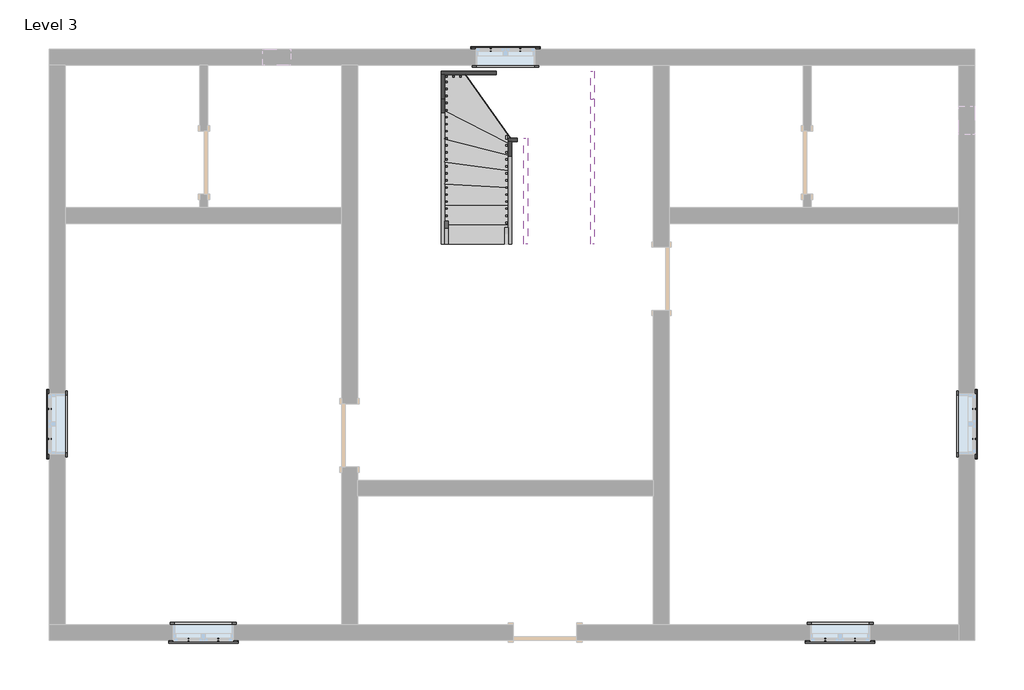
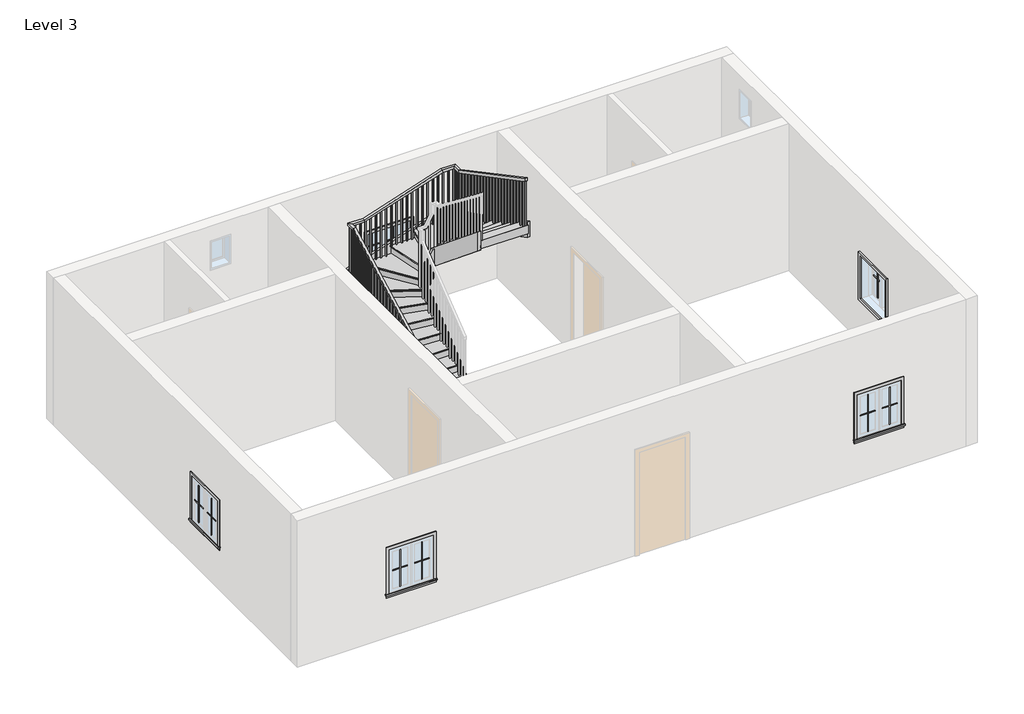
# One storey, part 2 of 2: 20 proxies, 8 members, 1 railing, 1 stair flight.
"""IFC4 building model written with IfcOpenShell, lengths in millimetres."""

from ifc_helpers import new_model, si_unit, frame, origin, place, context, project, spatial, polyline, outline, extrude, faceted_brep, transform, mapped, element, save
from components import muntin_pattern_2x2_muntin_pattern_2x2_b3fe6957, muntin_pattern_2x2_muntin_pattern_2x2_3e0ecaf2, trim_window_exterior_flat_with_sill_41619996, trim_window_interior_flat_picture_frame_51c85655, stair_flight_4b86e887

model = new_model("IFC4")

# Units and contexts
model_context = context("Model", 3, world=origin())
ifc_project = project(units=[si_unit("LENGTHUNIT", "METRE", prefix="MILLI")], contexts=[model_context])

# Site, building, storey
site = spatial("IfcSite", under=ifc_project)
building = spatial("IfcBuilding", under=site)
storey = spatial("IfcBuildingStorey", under=building, Name="Level 3", Elevation=3200.4)

# Proxies
placement = place(None, origin())
muntin_pattern_2x2_muntin_pattern_2x2_shape = muntin_pattern_2x2_muntin_pattern_2x2_b3fe6957(model_context)
element("IfcBuildingElementProxy", 1, Name="Muntin Pattern_2x2 : Muntin Pattern_2x2", ObjectType="Muntin Pattern_2x2 : Muntin Pattern_2x2", at=placement, inside=storey, context=model_context, shape_type="MappedRepresentation", body=[
    mapped(muntin_pattern_2x2_muntin_pattern_2x2_shape, transform((-7325.4390964, 833.891032, 4184.65), x_axis=(0.0, 1.0, 0.0), y_axis=(-1.0, 0.0, 0.0), z_axis=(0.0, 0.0, 1.0))),
])
element("IfcBuildingElementProxy", 2, Name="Muntin Pattern_2x2 : Muntin Pattern_2x2", ObjectType="Muntin Pattern_2x2 : Muntin Pattern_2x2", at=placement, inside=storey, context=model_context, shape_type="MappedRepresentation", body=[
    mapped(muntin_pattern_2x2_muntin_pattern_2x2_shape, transform((6006.3859036, 1262.516032, 4184.65), x_axis=(0.0, -1.0, 0.0), y_axis=(1.0, 0.0, 0.0), z_axis=(0.0, 0.0, 1.0))),
])
element("IfcBuildingElementProxy", 3, Name="Muntin Pattern_2x2 : Muntin Pattern_2x2", ObjectType="Muntin Pattern_2x2 : Muntin Pattern_2x2", at=placement, inside=storey, context=model_context, shape_type="MappedRepresentation", body=[
    mapped(muntin_pattern_2x2_muntin_pattern_2x2_shape, transform((-967.5015964, 6448.878532, 4184.65), x_axis=(1.0, 0.0, 0.0), y_axis=(0.0, 1.0, 0.0), z_axis=(0.0, 0.0, 1.0))),
])
element("IfcBuildingElementProxy", 4, Name="Muntin Pattern_2x2 : Muntin Pattern_2x2", ObjectType="Muntin Pattern_2x2 : Muntin Pattern_2x2", at=placement, inside=storey, context=model_context, shape_type="MappedRepresentation", body=[
    mapped(muntin_pattern_2x2_muntin_pattern_2x2_shape, transform((-4896.5640964, -2066.471468, 4184.65), x_axis=(-1.0, 0.0, 0.0), y_axis=(0.0, -1.0, 0.0), z_axis=(0.0, 0.0, 1.0))),
])
element("IfcBuildingElementProxy", 5, Name="Muntin Pattern_2x2 : Muntin Pattern_2x2", ObjectType="Muntin Pattern_2x2 : Muntin Pattern_2x2", at=placement, inside=storey, context=model_context, shape_type="MappedRepresentation", body=[
    mapped(muntin_pattern_2x2_muntin_pattern_2x2_shape, transform((4287.1234036, -2066.471468, 4184.65), x_axis=(-1.0, 0.0, 0.0), y_axis=(0.0, -1.0, 0.0), z_axis=(0.0, 0.0, 1.0))),
])
muntin_pattern_2x2_muntin_pattern_2x2_2_shape = muntin_pattern_2x2_muntin_pattern_2x2_3e0ecaf2(model_context)
element("IfcBuildingElementProxy", 6, Name="Muntin Pattern_2x2 : Muntin Pattern_2x2", ObjectType="Muntin Pattern_2x2 : Muntin Pattern_2x2", at=placement, inside=storey, context=model_context, shape_type="MappedRepresentation", body=[
    mapped(muntin_pattern_2x2_muntin_pattern_2x2_2_shape, transform((-7325.4390964, 1262.516032, 4184.65), x_axis=(0.0, -1.0, 0.0), y_axis=(1.0, 0.0, 0.0), z_axis=(0.0, 0.0, 1.0))),
])
element("IfcBuildingElementProxy", 7, Name="Muntin Pattern_2x2 : Muntin Pattern_2x2", ObjectType="Muntin Pattern_2x2 : Muntin Pattern_2x2", at=placement, inside=storey, context=model_context, shape_type="MappedRepresentation", body=[
    mapped(muntin_pattern_2x2_muntin_pattern_2x2_2_shape, transform((6006.3859036, 833.891032, 4184.65), x_axis=(0.0, 1.0, 0.0), y_axis=(-1.0, 0.0, 0.0), z_axis=(0.0, 0.0, 1.0))),
])
element("IfcBuildingElementProxy", 8, Name="Muntin Pattern_2x2 : Muntin Pattern_2x2", ObjectType="Muntin Pattern_2x2 : Muntin Pattern_2x2", at=placement, inside=storey, context=model_context, shape_type="MappedRepresentation", body=[
    mapped(muntin_pattern_2x2_muntin_pattern_2x2_2_shape, transform((-538.8765964, 6448.878532, 4184.65), x_axis=(-1.0, 0.0, 0.0), y_axis=(0.0, -1.0, 0.0), z_axis=(0.0, 0.0, 1.0))),
])
element("IfcBuildingElementProxy", 9, Name="Muntin Pattern_2x2 : Muntin Pattern_2x2", ObjectType="Muntin Pattern_2x2 : Muntin Pattern_2x2", at=placement, inside=storey, context=model_context, shape_type="MappedRepresentation", body=[
    mapped(muntin_pattern_2x2_muntin_pattern_2x2_2_shape, transform((-5325.1890964, -2066.471468, 4184.65), x_axis=(1.0, 0.0, 0.0), y_axis=(0.0, 1.0, 0.0), z_axis=(0.0, 0.0, 1.0))),
])
element("IfcBuildingElementProxy", 10, Name="Muntin Pattern_2x2 : Muntin Pattern_2x2", ObjectType="Muntin Pattern_2x2 : Muntin Pattern_2x2", at=placement, inside=storey, context=model_context, shape_type="MappedRepresentation", body=[
    mapped(muntin_pattern_2x2_muntin_pattern_2x2_2_shape, transform((3858.4984036, -2066.471468, 4184.65), x_axis=(1.0, 0.0, 0.0), y_axis=(0.0, 1.0, 0.0), z_axis=(0.0, 0.0, 1.0))),
])
trim_window_exterior_flat_with_sill_shape = trim_window_exterior_flat_with_sill_41619996(model_context)
element("IfcBuildingElementProxy", 11, Name="Trim-Window-Exterior-Flat : with Sill", ObjectType="Trim-Window-Exterior-Flat : with Sill", at=placement, inside=storey, context=model_context, shape_type="MappedRepresentation", body=[
    mapped(trim_window_exterior_flat_with_sill_shape, transform((-7334.9640964, 1048.203532, 5029.2), x_axis=(0.0, -1.0, 0.0), y_axis=(0.0, 0.0, 1.0), z_axis=(-1.0, 0.0, 0.0))),
])
element("IfcBuildingElementProxy", 12, Name="Trim-Window-Exterior-Flat : with Sill", ObjectType="Trim-Window-Exterior-Flat : with Sill", at=placement, inside=storey, context=model_context, shape_type="MappedRepresentation", body=[
    mapped(trim_window_exterior_flat_with_sill_shape, transform((6015.9109036, 1048.203532, 5029.2), x_axis=(0.0, 1.0, 0.0), y_axis=(0.0, 0.0, 1.0), z_axis=(1.0, 0.0, 0.0))),
])
element("IfcBuildingElementProxy", 13, Name="Trim-Window-Exterior-Flat : with Sill", ObjectType="Trim-Window-Exterior-Flat : with Sill", at=placement, inside=storey, context=model_context, shape_type="MappedRepresentation", body=[
    mapped(trim_window_exterior_flat_with_sill_shape, transform((-753.1890964, 6458.403532, 5029.2), x_axis=(-1.0, 0.0, 0.0), y_axis=(0.0, 0.0, 1.0), z_axis=(0.0, 1.0, 0.0))),
])
element("IfcBuildingElementProxy", 14, Name="Trim-Window-Exterior-Flat : with Sill", ObjectType="Trim-Window-Exterior-Flat : with Sill", at=placement, inside=storey, context=model_context, shape_type="MappedRepresentation", body=[
    mapped(trim_window_exterior_flat_with_sill_shape, transform((-5110.8765964, -2075.996468, 5029.2), x_axis=(1.0, 0.0, 0.0), y_axis=(0.0, 0.0, 1.0), z_axis=(0.0, -1.0, 0.0))),
])
element("IfcBuildingElementProxy", 15, Name="Trim-Window-Exterior-Flat : with Sill", ObjectType="Trim-Window-Exterior-Flat : with Sill", at=placement, inside=storey, context=model_context, shape_type="MappedRepresentation", body=[
    mapped(trim_window_exterior_flat_with_sill_shape, transform((4072.8109036, -2075.996468, 5029.2), x_axis=(1.0, 0.0, 0.0), y_axis=(0.0, 0.0, 1.0), z_axis=(0.0, -1.0, 0.0))),
])
trim_window_interior_flat_picture_frame_shape = trim_window_interior_flat_picture_frame_51c85655(model_context)
element("IfcBuildingElementProxy", 16, Name="Trim-Window-Interior-Flat : Picture Frame", ObjectType="Trim-Window-Interior-Flat : Picture Frame", at=placement, inside=storey, context=model_context, shape_type="MappedRepresentation", body=[
    mapped(trim_window_interior_flat_picture_frame_shape, transform((-7106.3640964, 1048.203532, 5029.2), x_axis=(0.0, 1.0, 0.0), y_axis=(0.0, 0.0, 1.0), z_axis=(1.0, 0.0, 0.0))),
])
element("IfcBuildingElementProxy", 17, Name="Trim-Window-Interior-Flat : Picture Frame", ObjectType="Trim-Window-Interior-Flat : Picture Frame", at=placement, inside=storey, context=model_context, shape_type="MappedRepresentation", body=[
    mapped(trim_window_interior_flat_picture_frame_shape, transform((5787.3109036, 1048.203532, 5029.2), x_axis=(0.0, -1.0, 0.0), y_axis=(0.0, 0.0, 1.0), z_axis=(-1.0, 0.0, 0.0))),
])
element("IfcBuildingElementProxy", 18, Name="Trim-Window-Interior-Flat : Picture Frame", ObjectType="Trim-Window-Interior-Flat : Picture Frame", at=placement, inside=storey, context=model_context, shape_type="MappedRepresentation", body=[
    mapped(trim_window_interior_flat_picture_frame_shape, transform((-753.1890964, 6229.803532, 5029.2), x_axis=(1.0, 0.0, 0.0), y_axis=(0.0, 0.0, 1.0), z_axis=(0.0, -1.0, 0.0))),
])
element("IfcBuildingElementProxy", 19, Name="Trim-Window-Interior-Flat : Picture Frame", ObjectType="Trim-Window-Interior-Flat : Picture Frame", at=placement, inside=storey, context=model_context, shape_type="MappedRepresentation", body=[
    mapped(trim_window_interior_flat_picture_frame_shape, transform((-5110.8765964, -1847.396468, 5029.2), x_axis=(-1.0, 0.0, 0.0), y_axis=(0.0, 0.0, 1.0), z_axis=(0.0, 1.0, 0.0))),
])
element("IfcBuildingElementProxy", 20, Name="Trim-Window-Interior-Flat : Picture Frame", ObjectType="Trim-Window-Interior-Flat : Picture Frame", at=placement, inside=storey, context=model_context, shape_type="MappedRepresentation", body=[
    mapped(trim_window_interior_flat_picture_frame_shape, transform((4072.8109036, -1847.396468, 5029.2), x_axis=(-1.0, 0.0, 0.0), y_axis=(0.0, 0.0, 1.0), z_axis=(0.0, 1.0, 0.0))),
])

# Members
element("IfcMember", 21, ObjectType="Stringer - 2\" Width", at=placement, inside=storey, context=model_context, shape_type="SweptSolid", body=[
    extrude(outline(polyline([(3647.9718401, 3200.4), (3647.9718401, 3430.039954), (5735.3890318, 4505.7956453), (5735.3890318, 4162.900629), (3867.7341577, 3200.4), (3647.9718401, 3200.4)])), frame((-1680.2890964, 0.0, 0.0), z_axis=(1.0, 0.0, 0.0), x_axis=(0.0, 1.0, 0.0)), (0.0, 0.0, 1.0), 50.8),
])
element("IfcMember", 22, ObjectType="Stringer - 2\" Width", at=placement, inside=storey, context=model_context, shape_type="SweptSolid", body=[
    extrude(outline(polyline([(-1629.4890964, 5735.3890318), (-1680.2890964, 5735.3890318), (-1680.2890964, 6090.103532), (-1629.4890964, 6090.103532), (-1629.4890964, 5735.3890318)])), frame((0.0, 0.0, 4162.900629), z_axis=(0.0, 0.0, 1.0), x_axis=(1.0, 0.0, 0.0)), (0.0, 0.0, 1.0), 342.8950162),
])
element("IfcMember", 23, ObjectType="Stringer - 2\" Width", at=placement, inside=storey, context=model_context, shape_type="SweptSolid", body=[
    extrude(outline(polyline([(4489.4952212, -1680.2890964), (4200.9956453, -1680.2890964), (4200.9956453, -1510.7666134), (4839.3682298, 478.7109036), (5170.3972697, 478.7109036), (5170.3972697, 441.7307863), (4489.4952212, -1680.2890964)])), frame((0.0, 6090.103532, 0.0), z_axis=(0.0, 1.0, 0.0), x_axis=(0.0, 0.0, 1.0)), (0.0, 0.0, 1.0), 50.8),
])
element("IfcMember", 24, ObjectType="Stringer - 2\" Width", at=placement, inside=storey, context=model_context, shape_type="SweptSolid", body=[
    extrude(outline(polyline([(478.7109036, 6140.903532), (529.5109036, 6140.903532), (529.5109036, 5735.3890318), (478.7109036, 5735.3890318), (478.7109036, 6140.903532)])), frame((0.0, 0.0, 4850.2904473), z_axis=(0.0, 0.0, 1.0), x_axis=(1.0, 0.0, 0.0)), (0.0, 0.0, 1.0), 320.1068224),
])
element("IfcMember", 25, ObjectType="Stringer - 2\" Width", at=placement, inside=storey, context=model_context, shape_type="SweptSolid", body=[
    extrude(outline(polyline([(5735.3890318, 5170.3972697), (5735.3890318, 4850.2904473), (3647.9718401, 5926.0461385), (3647.9718401, 6246.1529609), (5735.3890318, 5170.3972697)])), frame((478.7109036, 0.0, 0.0), z_axis=(1.0, 0.0, 0.0), x_axis=(0.0, 1.0, 0.0)), (0.0, 0.0, 1.0), 50.8),
])
element("IfcMember", 26, ObjectType="Stringer - 2\" Width", at=placement, inside=storey, context=model_context, shape_type="SweptSolid", body=[
    extrude(outline(polyline([(3647.9718401, 3200.4), (3647.9718401, 3376.5764461), (5124.903532, 4580.818648), (5124.903532, 4187.5410923), (3914.2334847, 3200.4), (3647.9718401, 3200.4)])), frame((-715.0890964, 0.0, 0.0), z_axis=(1.0, 0.0, 0.0), x_axis=(0.0, 1.0, 0.0)), (0.0, 0.0, 1.0), 50.8),
])
element("IfcMember", 27, ObjectType="Stringer - 2\" Width", at=placement, inside=storey, context=model_context, shape_type="SweptSolid", body=[
    extrude(outline(polyline([(4773.6682978, -715.0890964), (4228.9617647, -715.0890964), (4228.9617647, -680.846879), (4560.865107, -486.4890964), (5126.5409689, -486.4890964), (5126.5409689, -508.4519789), (4773.6682978, -715.0890964)])), frame((0.0, 5124.903532, 0.0), z_axis=(0.0, 1.0, 0.0), x_axis=(0.0, 0.0, 1.0)), (0.0, 0.0, 1.0), 50.8),
])
element("IfcMember", 28, ObjectType="Stringer - 2\" Width", at=placement, inside=storey, context=model_context, shape_type="SweptSolid", body=[
    extrude(outline(polyline([(5175.703532, 5126.5409689), (5175.703532, 4733.2634131), (3647.9718401, 5978.9262875), (3647.9718401, 6372.2038432), (5175.703532, 5126.5409689)])), frame((-486.4890964, 0.0, 0.0), z_axis=(1.0, 0.0, 0.0), x_axis=(0.0, 1.0, 0.0)), (0.0, 0.0, 1.0), 50.8),
])

# Railing
element("IfcRailing", 29, ObjectType="Handrail - Rectangular", at=placement, inside=storey, context=model_context, shape_type="SolidModel", body=[
    faceted_brep([(-1629.4890964, 3647.9718401, 4284.1333333), (-1629.4890964, 3647.9718401, 4226.6742652), (-1578.6890964, 3647.9718401, 4226.6742652), (-1578.6890964, 3647.9718401, 4284.1333333), (-1629.4890964, 5905.6969022, 5477.4239201), (-1629.4890964, 5918.2959667, 5426.6239201), (-1578.6890964, 5918.2959667, 5426.6239201), (-1578.6890964, 5905.6969022, 5477.4239201), (-1629.4890964, 6090.103532, 5477.4239201), (-1629.4890964, 6090.103532, 5426.6239201), (-1578.6890964, 6039.303532, 5426.6239201), (-1578.6890964, 6039.303532, 5477.4239201), (-1342.1772142, 6090.103532, 5477.4239201), (-1334.2266381, 6090.103532, 5426.6239201), (-1334.2266381, 6039.303532, 5426.6239201), (-1342.1772142, 6039.303532, 5477.4239201), (191.3990215, 6090.103532, 5969.5094132), (199.3495976, 6090.103532, 5918.7094132), (199.3495976, 6039.303532, 5918.7094132), (191.3990215, 6039.303532, 5969.5094132), (478.7109036, 6090.103532, 5969.5094132), (478.7109036, 6090.103532, 5918.7094132), (427.9109036, 6039.303532, 5918.7094132), (427.9109036, 6039.303532, 5969.5094132), (478.7109036, 5905.6969022, 5969.5094132), (478.7109036, 5893.0978376, 5918.7094132), (427.9109036, 5893.0978376, 5918.7094132), (427.9109036, 5905.6969022, 5969.5094132), (478.7109036, 3647.9718401, 7162.8), (427.9109036, 3647.9718401, 7162.8), (427.9109036, 3647.9718401, 7105.3409318), (478.7109036, 3647.9718401, 7105.3409318)], [[[0, 1, 2, 3]], [[1, 0, 4, 5]], [[2, 1, 5, 6]], [[3, 2, 6, 7]], [[0, 3, 7, 4]], [[5, 4, 8, 9]], [[6, 5, 9, 10]], [[7, 6, 10, 11]], [[4, 7, 11, 8]], [[9, 8, 12, 13]], [[10, 9, 13, 14]], [[11, 10, 14, 15]], [[8, 11, 15, 12]], [[13, 12, 16, 17]], [[14, 13, 17, 18]], [[15, 14, 18, 19]], [[12, 15, 19, 16]], [[17, 16, 20, 21]], [[18, 17, 21, 22]], [[19, 18, 22, 23]], [[16, 19, 23, 20]], [[21, 20, 24, 25]], [[22, 21, 25, 26]], [[23, 22, 26, 27]], [[20, 23, 27, 24]], [[28, 29, 30, 31]], [[25, 24, 28, 31]], [[26, 25, 31, 30]], [[27, 26, 30, 29]], [[24, 27, 29, 28]]]),
    extrude(outline(polyline([(3737.428532, 7058.0597858), (3737.428532, 6079.0666667), (3718.378532, 6079.0666667), (3718.378532, 7068.1284102), (3737.428532, 7058.0597858)])), frame((443.7859036, 0.0, 0.0), z_axis=(1.0, 0.0, 0.0), x_axis=(0.0, 1.0, 0.0)), (0.0, 0.0, 1.0), 19.05),
    extrude(outline(polyline([(3839.028532, 7004.3604556), (3839.028532, 6079.0666667), (3819.978532, 6079.0666667), (3819.978532, 7014.42908), (3839.028532, 7004.3604556)])), frame((443.7859036, 0.0, 0.0), z_axis=(1.0, 0.0, 0.0), x_axis=(0.0, 1.0, 0.0)), (0.0, 0.0, 1.0), 19.05),
    extrude(outline(polyline([(3940.628532, 6950.6611254), (3940.628532, 5909.7333333), (3921.578532, 5909.7333333), (3921.578532, 6960.7297498), (3940.628532, 6950.6611254)])), frame((443.7859036, 0.0, 0.0), z_axis=(1.0, 0.0, 0.0), x_axis=(0.0, 1.0, 0.0)), (0.0, 0.0, 1.0), 19.05),
    extrude(outline(polyline([(4042.228532, 6896.9617952), (4042.228532, 5909.7333333), (4023.178532, 5909.7333333), (4023.178532, 6907.0304196), (4042.228532, 6896.9617952)])), frame((443.7859036, 0.0, 0.0), z_axis=(1.0, 0.0, 0.0), x_axis=(0.0, 1.0, 0.0)), (0.0, 0.0, 1.0), 19.05),
    extrude(outline(polyline([(4143.828532, 6843.262465), (4143.828532, 5909.7333333), (4124.778532, 5909.7333333), (4124.778532, 6853.3310894), (4143.828532, 6843.262465)])), frame((443.7859036, 0.0, 0.0), z_axis=(1.0, 0.0, 0.0), x_axis=(0.0, 1.0, 0.0)), (0.0, 0.0, 1.0), 19.05),
    extrude(outline(polyline([(4245.428532, 6789.5631348), (4245.428532, 5740.4), (4226.378532, 5740.4), (4226.378532, 6799.6317592), (4245.428532, 6789.5631348)])), frame((443.7859036, 0.0, 0.0), z_axis=(1.0, 0.0, 0.0), x_axis=(0.0, 1.0, 0.0)), (0.0, 0.0, 1.0), 19.05),
    extrude(outline(polyline([(4347.028532, 6735.8638046), (4347.028532, 5740.4), (4327.978532, 5740.4), (4327.978532, 6745.932429), (4347.028532, 6735.8638046)])), frame((443.7859036, 0.0, 0.0), z_axis=(1.0, 0.0, 0.0), x_axis=(0.0, 1.0, 0.0)), (0.0, 0.0, 1.0), 19.05),
    extrude(outline(polyline([(4448.628532, 6682.1644744), (4448.628532, 5740.4), (4429.578532, 5740.4), (4429.578532, 6692.2330988), (4448.628532, 6682.1644744)])), frame((443.7859036, 0.0, 0.0), z_axis=(1.0, 0.0, 0.0), x_axis=(0.0, 1.0, 0.0)), (0.0, 0.0, 1.0), 19.05),
    extrude(outline(polyline([(4550.228532, 6628.4651442), (4550.228532, 5571.0666667), (4531.178532, 5571.0666667), (4531.178532, 6638.5337686), (4550.228532, 6628.4651442)])), frame((443.7859036, 0.0, 0.0), z_axis=(1.0, 0.0, 0.0), x_axis=(0.0, 1.0, 0.0)), (0.0, 0.0, 1.0), 19.05),
    extrude(outline(polyline([(4651.828532, 6574.765814), (4651.828532, 5571.0666667), (4632.778532, 5571.0666667), (4632.778532, 6584.8344384), (4651.828532, 6574.765814)])), frame((443.7859036, 0.0, 0.0), z_axis=(1.0, 0.0, 0.0), x_axis=(0.0, 1.0, 0.0)), (0.0, 0.0, 1.0), 19.05),
    extrude(outline(polyline([(4753.428532, 6521.0664838), (4753.428532, 5571.0666667), (4734.378532, 5571.0666667), (4734.378532, 6531.1351082), (4753.428532, 6521.0664838)])), frame((443.7859036, 0.0, 0.0), z_axis=(1.0, 0.0, 0.0), x_axis=(0.0, 1.0, 0.0)), (0.0, 0.0, 1.0), 19.05),
    extrude(outline(polyline([(4855.028532, 6467.3671536), (4855.028532, 5401.7333333), (4835.978532, 5401.7333333), (4835.978532, 6477.435778), (4855.028532, 6467.3671536)])), frame((443.7859036, 0.0, 0.0), z_axis=(1.0, 0.0, 0.0), x_axis=(0.0, 1.0, 0.0)), (0.0, 0.0, 1.0), 19.05),
    extrude(outline(polyline([(4956.628532, 6413.6678234), (4956.628532, 5401.7333333), (4937.578532, 5401.7333333), (4937.578532, 6423.7364478), (4956.628532, 6413.6678234)])), frame((443.7859036, 0.0, 0.0), z_axis=(1.0, 0.0, 0.0), x_axis=(0.0, 1.0, 0.0)), (0.0, 0.0, 1.0), 19.05),
    extrude(outline(polyline([(5058.228532, 6359.9684932), (5058.228532, 5401.7333333), (5039.178532, 5401.7333333), (5039.178532, 6370.0371176), (5058.228532, 6359.9684932)])), frame((443.7859036, 0.0, 0.0), z_axis=(1.0, 0.0, 0.0), x_axis=(0.0, 1.0, 0.0)), (0.0, 0.0, 1.0), 19.05),
    extrude(outline(polyline([(5159.828532, 6306.269163), (5159.828532, 5401.7333333), (5140.778532, 5401.7333333), (5140.778532, 6316.3377874), (5159.828532, 6306.269163)])), frame((443.7859036, 0.0, 0.0), z_axis=(1.0, 0.0, 0.0), x_axis=(0.0, 1.0, 0.0)), (0.0, 0.0, 1.0), 19.05),
    extrude(outline(polyline([(5261.428532, 6252.5698328), (5261.428532, 5232.4), (5242.378532, 5232.4), (5242.378532, 6262.6384572), (5261.428532, 6252.5698328)])), frame((443.7859036, 0.0, 0.0), z_axis=(1.0, 0.0, 0.0), x_axis=(0.0, 1.0, 0.0)), (0.0, 0.0, 1.0), 19.05),
    extrude(outline(polyline([(5363.028532, 6198.8705026), (5363.028532, 5232.4), (5343.978532, 5232.4), (5343.978532, 6208.939127), (5363.028532, 6198.8705026)])), frame((443.7859036, 0.0, 0.0), z_axis=(1.0, 0.0, 0.0), x_axis=(0.0, 1.0, 0.0)), (0.0, 0.0, 1.0), 19.05),
    extrude(outline(polyline([(5464.628532, 6145.1711724), (5464.628532, 5232.4), (5445.578532, 5232.4), (5445.578532, 6155.2397968), (5464.628532, 6145.1711724)])), frame((443.7859036, 0.0, 0.0), z_axis=(1.0, 0.0, 0.0), x_axis=(0.0, 1.0, 0.0)), (0.0, 0.0, 1.0), 19.05),
    extrude(outline(polyline([(5566.228532, 6091.4718422), (5566.228532, 5232.4), (5547.178532, 5232.4), (5547.178532, 6101.5404666), (5566.228532, 6091.4718422)])), frame((443.7859036, 0.0, 0.0), z_axis=(1.0, 0.0, 0.0), x_axis=(0.0, 1.0, 0.0)), (0.0, 0.0, 1.0), 19.05),
    extrude(outline(polyline([(5667.828532, 6037.772512), (5667.828532, 5063.0666667), (5648.778532, 5063.0666667), (5648.778532, 6047.8411364), (5667.828532, 6037.772512)])), frame((443.7859036, 0.0, 0.0), z_axis=(1.0, 0.0, 0.0), x_axis=(0.0, 1.0, 0.0)), (0.0, 0.0, 1.0), 19.05),
    extrude(outline(polyline([(5769.428532, 5984.0731818), (5769.428532, 5063.0666667), (5750.378532, 5063.0666667), (5750.378532, 5994.1418062), (5769.428532, 5984.0731818)])), frame((443.7859036, 0.0, 0.0), z_axis=(1.0, 0.0, 0.0), x_axis=(0.0, 1.0, 0.0)), (0.0, 0.0, 1.0), 19.05),
    extrude(outline(polyline([(5871.028532, 5930.3738516), (5871.028532, 5063.0666667), (5851.978532, 5063.0666667), (5851.978532, 5940.442476), (5871.028532, 5930.3738516)])), frame((443.7859036, 0.0, 0.0), z_axis=(1.0, 0.0, 0.0), x_axis=(0.0, 1.0, 0.0)), (0.0, 0.0, 1.0), 19.05),
    extrude(outline(polyline([(462.8359036, 5972.628532), (462.8359036, 5953.578532), (443.7859036, 5953.578532), (443.7859036, 5972.628532), (462.8359036, 5972.628532)])), frame((0.0, 0.0, 5063.0666667), z_axis=(0.0, 0.0, 1.0), x_axis=(1.0, 0.0, 0.0)), (0.0, 0.0, 1.0), 855.6427466),
    extrude(outline(polyline([(418.3859036, 6074.228532), (437.4359036, 6074.228532), (437.4359036, 6055.178532), (418.3859036, 6055.178532), (418.3859036, 6074.228532)])), frame((0.0, 0.0, 5063.0666667), z_axis=(0.0, 0.0, 1.0), x_axis=(1.0, 0.0, 0.0)), (0.0, 0.0, 1.0), 855.6427466),
    extrude(outline(polyline([(316.7859036, 6074.228532), (335.8359036, 6074.228532), (335.8359036, 6055.178532), (316.7859036, 6055.178532), (316.7859036, 6074.228532)])), frame((0.0, 0.0, 5063.0666667), z_axis=(0.0, 0.0, 1.0), x_axis=(1.0, 0.0, 0.0)), (0.0, 0.0, 1.0), 855.6427466),
    extrude(outline(polyline([(215.1859036, 6074.228532), (234.2359036, 6074.228532), (234.2359036, 6055.178532), (215.1859036, 6055.178532), (215.1859036, 6074.228532)])), frame((0.0, 0.0, 5063.0666667), z_axis=(0.0, 0.0, 1.0), x_axis=(1.0, 0.0, 0.0)), (0.0, 0.0, 1.0), 855.6427466),
    extrude(outline(polyline([(5891.1900316, 113.5859036), (4893.7333333, 113.5859036), (4893.7333333, 132.6359036), (5897.3026907, 132.6359036), (5891.1900316, 113.5859036)])), frame((0.0, 6055.178532, 0.0), z_axis=(0.0, 1.0, 0.0), x_axis=(0.0, 0.0, 1.0)), (0.0, 0.0, 1.0), 19.05),
    extrude(outline(polyline([(5858.5891834, 11.9859036), (4893.7333333, 11.9859036), (4893.7333333, 31.0359036), (5864.7018425, 31.0359036), (5858.5891834, 11.9859036)])), frame((0.0, 6055.178532, 0.0), z_axis=(0.0, 1.0, 0.0), x_axis=(0.0, 0.0, 1.0)), (0.0, 0.0, 1.0), 19.05),
    extrude(outline(polyline([(5825.9883352, -89.6140964), (4893.7333333, -89.6140964), (4893.7333333, -70.5640964), (5832.1009942, -70.5640964), (5825.9883352, -89.6140964)])), frame((0.0, 6055.178532, 0.0), z_axis=(0.0, 1.0, 0.0), x_axis=(0.0, 0.0, 1.0)), (0.0, 0.0, 1.0), 19.05),
    extrude(outline(polyline([(5793.387487, -191.2140964), (4893.7333333, -191.2140964), (4893.7333333, -172.1640964), (5799.500146, -172.1640964), (5793.387487, -191.2140964)])), frame((0.0, 6055.178532, 0.0), z_axis=(0.0, 1.0, 0.0), x_axis=(0.0, 0.0, 1.0)), (0.0, 0.0, 1.0), 19.05),
    extrude(outline(polyline([(5760.7866387, -292.8140964), (4893.7333333, -292.8140964), (4893.7333333, -273.7640964), (5766.8992978, -273.7640964), (5760.7866387, -292.8140964)])), frame((0.0, 6055.178532, 0.0), z_axis=(0.0, 1.0, 0.0), x_axis=(0.0, 0.0, 1.0)), (0.0, 0.0, 1.0), 19.05),
    extrude(outline(polyline([(5728.1857905, -394.4140964), (4724.4, -394.4140964), (4724.4, -375.3640964), (5734.2984495, -375.3640964), (5728.1857905, -394.4140964)])), frame((0.0, 6055.178532, 0.0), z_axis=(0.0, 1.0, 0.0), x_axis=(0.0, 0.0, 1.0)), (0.0, 0.0, 1.0), 19.05),
    extrude(outline(polyline([(5695.5849423, -496.0140964), (4724.4, -496.0140964), (4724.4, -476.9640964), (5701.6976013, -476.9640964), (5695.5849423, -496.0140964)])), frame((0.0, 6055.178532, 0.0), z_axis=(0.0, 1.0, 0.0), x_axis=(0.0, 0.0, 1.0)), (0.0, 0.0, 1.0), 19.05),
    extrude(outline(polyline([(5662.984094, -597.6140964), (4724.4, -597.6140964), (4724.4, -578.5640964), (5669.0967531, -578.5640964), (5662.984094, -597.6140964)])), frame((0.0, 6055.178532, 0.0), z_axis=(0.0, 1.0, 0.0), x_axis=(0.0, 0.0, 1.0)), (0.0, 0.0, 1.0), 19.05),
    extrude(outline(polyline([(5630.3832458, -699.2140964), (4724.4, -699.2140964), (4724.4, -680.1640964), (5636.4959049, -680.1640964), (5630.3832458, -699.2140964)])), frame((0.0, 6055.178532, 0.0), z_axis=(0.0, 1.0, 0.0), x_axis=(0.0, 0.0, 1.0)), (0.0, 0.0, 1.0), 19.05),
    extrude(outline(polyline([(5597.7823976, -800.8140964), (4724.4, -800.8140964), (4724.4, -781.7640964), (5603.8950566, -781.7640964), (5597.7823976, -800.8140964)])), frame((0.0, 6055.178532, 0.0), z_axis=(0.0, 1.0, 0.0), x_axis=(0.0, 0.0, 1.0)), (0.0, 0.0, 1.0), 19.05),
    extrude(outline(polyline([(5565.1815494, -902.4140964), (4555.0666667, -902.4140964), (4555.0666667, -883.3640964), (5571.2942084, -883.3640964), (5565.1815494, -902.4140964)])), frame((0.0, 6055.178532, 0.0), z_axis=(0.0, 1.0, 0.0), x_axis=(0.0, 0.0, 1.0)), (0.0, 0.0, 1.0), 19.05),
    extrude(outline(polyline([(5532.5807011, -1004.0140964), (4555.0666667, -1004.0140964), (4555.0666667, -984.9640964), (5538.6933602, -984.9640964), (5532.5807011, -1004.0140964)])), frame((0.0, 6055.178532, 0.0), z_axis=(0.0, 1.0, 0.0), x_axis=(0.0, 0.0, 1.0)), (0.0, 0.0, 1.0), 19.05),
    extrude(outline(polyline([(5499.9798529, -1105.6140964), (4555.0666667, -1105.6140964), (4555.0666667, -1086.5640964), (5506.092512, -1086.5640964), (5499.9798529, -1105.6140964)])), frame((0.0, 6055.178532, 0.0), z_axis=(0.0, 1.0, 0.0), x_axis=(0.0, 0.0, 1.0)), (0.0, 0.0, 1.0), 19.05),
    extrude(outline(polyline([(5467.3790047, -1207.2140964), (4555.0666667, -1207.2140964), (4555.0666667, -1188.1640964), (5473.4916637, -1188.1640964), (5467.3790047, -1207.2140964)])), frame((0.0, 6055.178532, 0.0), z_axis=(0.0, 1.0, 0.0), x_axis=(0.0, 0.0, 1.0)), (0.0, 0.0, 1.0), 19.05),
    extrude(outline(polyline([(5434.7781565, -1308.8140964), (4555.0666667, -1308.8140964), (4555.0666667, -1289.7640964), (5440.8908155, -1289.7640964), (5434.7781565, -1308.8140964)])), frame((0.0, 6055.178532, 0.0), z_axis=(0.0, 1.0, 0.0), x_axis=(0.0, 0.0, 1.0)), (0.0, 0.0, 1.0), 19.05),
    extrude(outline(polyline([(-1410.4140964, 6074.228532), (-1391.3640964, 6074.228532), (-1391.3640964, 6055.178532), (-1410.4140964, 6055.178532), (-1410.4140964, 6074.228532)])), frame((0.0, 0.0, 4385.7333333), z_axis=(0.0, 0.0, 1.0), x_axis=(1.0, 0.0, 0.0)), (0.0, 0.0, 1.0), 1040.8905868),
    extrude(outline(polyline([(-1512.0140964, 6074.228532), (-1492.9640964, 6074.228532), (-1492.9640964, 6055.178532), (-1512.0140964, 6055.178532), (-1512.0140964, 6074.228532)])), frame((0.0, 0.0, 4385.7333333), z_axis=(0.0, 0.0, 1.0), x_axis=(1.0, 0.0, 0.0)), (0.0, 0.0, 1.0), 1040.8905868),
    extrude(outline(polyline([(-1613.6140964, 5975.2468401), (-1613.6140964, 5994.2968401), (-1594.5640964, 5994.2968401), (-1594.5640964, 5975.2468401), (-1613.6140964, 5975.2468401)])), frame((0.0, 0.0, 4385.7333333), z_axis=(0.0, 0.0, 1.0), x_axis=(1.0, 0.0, 0.0)), (0.0, 0.0, 1.0), 1040.8905868),
    extrude(outline(polyline([(5892.6968401, 5413.0938418), (5892.6968401, 4385.7333333), (5873.6468401, 4385.7333333), (5873.6468401, 5403.0252174), (5892.6968401, 5413.0938418)])), frame((-1613.6140964, 0.0, 0.0), z_axis=(1.0, 0.0, 0.0), x_axis=(0.0, 1.0, 0.0)), (0.0, 0.0, 1.0), 19.05),
    extrude(outline(polyline([(5791.0968401, 5359.3945116), (5791.0968401, 4385.7333333), (5772.0468401, 4385.7333333), (5772.0468401, 5349.3258872), (5791.0968401, 5359.3945116)])), frame((-1613.6140964, 0.0, 0.0), z_axis=(1.0, 0.0, 0.0), x_axis=(0.0, 1.0, 0.0)), (0.0, 0.0, 1.0), 19.05),
    extrude(outline(polyline([(5689.4968401, 5305.6951814), (5689.4968401, 4385.7333333), (5670.4468401, 4385.7333333), (5670.4468401, 5295.626557), (5689.4968401, 5305.6951814)])), frame((-1613.6140964, 0.0, 0.0), z_axis=(1.0, 0.0, 0.0), x_axis=(0.0, 1.0, 0.0)), (0.0, 0.0, 1.0), 19.05),
    extrude(outline(polyline([(5587.8968401, 5251.9958512), (5587.8968401, 4385.7333333), (5568.8468401, 4385.7333333), (5568.8468401, 5241.9272268), (5587.8968401, 5251.9958512)])), frame((-1613.6140964, 0.0, 0.0), z_axis=(1.0, 0.0, 0.0), x_axis=(0.0, 1.0, 0.0)), (0.0, 0.0, 1.0), 19.05),
    extrude(outline(polyline([(5486.2968401, 5198.296521), (5486.2968401, 4216.4), (5467.2468401, 4216.4), (5467.2468401, 5188.2278966), (5486.2968401, 5198.296521)])), frame((-1613.6140964, 0.0, 0.0), z_axis=(1.0, 0.0, 0.0), x_axis=(0.0, 1.0, 0.0)), (0.0, 0.0, 1.0), 19.05),
    extrude(outline(polyline([(5384.6968401, 5144.5971908), (5384.6968401, 4216.4), (5365.6468401, 4216.4), (5365.6468401, 5134.5285664), (5384.6968401, 5144.5971908)])), frame((-1613.6140964, 0.0, 0.0), z_axis=(1.0, 0.0, 0.0), x_axis=(0.0, 1.0, 0.0)), (0.0, 0.0, 1.0), 19.05),
    extrude(outline(polyline([(5283.0968401, 5090.8978606), (5283.0968401, 4216.4), (5264.0468401, 4216.4), (5264.0468401, 5080.8292362), (5283.0968401, 5090.8978606)])), frame((-1613.6140964, 0.0, 0.0), z_axis=(1.0, 0.0, 0.0), x_axis=(0.0, 1.0, 0.0)), (0.0, 0.0, 1.0), 19.05),
    extrude(outline(polyline([(5181.4968401, 5037.1985304), (5181.4968401, 4216.4), (5162.4468401, 4216.4), (5162.4468401, 5027.129906), (5181.4968401, 5037.1985304)])), frame((-1613.6140964, 0.0, 0.0), z_axis=(1.0, 0.0, 0.0), x_axis=(0.0, 1.0, 0.0)), (0.0, 0.0, 1.0), 19.05),
    extrude(outline(polyline([(5079.8968401, 4983.4992002), (5079.8968401, 4047.0666667), (5060.8468401, 4047.0666667), (5060.8468401, 4973.4305758), (5079.8968401, 4983.4992002)])), frame((-1613.6140964, 0.0, 0.0), z_axis=(1.0, 0.0, 0.0), x_axis=(0.0, 1.0, 0.0)), (0.0, 0.0, 1.0), 19.05),
    extrude(outline(polyline([(4978.2968401, 4929.79987), (4978.2968401, 4047.0666667), (4959.2468401, 4047.0666667), (4959.2468401, 4919.7312456), (4978.2968401, 4929.79987)])), frame((-1613.6140964, 0.0, 0.0), z_axis=(1.0, 0.0, 0.0), x_axis=(0.0, 1.0, 0.0)), (0.0, 0.0, 1.0), 19.05),
    extrude(outline(polyline([(4876.6968401, 4876.1005398), (4876.6968401, 4047.0666667), (4857.6468401, 4047.0666667), (4857.6468401, 4866.0319154), (4876.6968401, 4876.1005398)])), frame((-1613.6140964, 0.0, 0.0), z_axis=(1.0, 0.0, 0.0), x_axis=(0.0, 1.0, 0.0)), (0.0, 0.0, 1.0), 19.05),
    extrude(outline(polyline([(4775.0968401, 4822.4012096), (4775.0968401, 3877.7333333), (4756.0468401, 3877.7333333), (4756.0468401, 4812.3325852), (4775.0968401, 4822.4012096)])), frame((-1613.6140964, 0.0, 0.0), z_axis=(1.0, 0.0, 0.0), x_axis=(0.0, 1.0, 0.0)), (0.0, 0.0, 1.0), 19.05),
    extrude(outline(polyline([(4673.4968401, 4768.7018794), (4673.4968401, 3877.7333333), (4654.4468401, 3877.7333333), (4654.4468401, 4758.633255), (4673.4968401, 4768.7018794)])), frame((-1613.6140964, 0.0, 0.0), z_axis=(1.0, 0.0, 0.0), x_axis=(0.0, 1.0, 0.0)), (0.0, 0.0, 1.0), 19.05),
    extrude(outline(polyline([(4571.8968401, 4715.0025492), (4571.8968401, 3877.7333333), (4552.8468401, 3877.7333333), (4552.8468401, 4704.9339248), (4571.8968401, 4715.0025492)])), frame((-1613.6140964, 0.0, 0.0), z_axis=(1.0, 0.0, 0.0), x_axis=(0.0, 1.0, 0.0)), (0.0, 0.0, 1.0), 19.05),
    extrude(outline(polyline([(4470.2968401, 4661.303219), (4470.2968401, 3708.4), (4451.2468401, 3708.4), (4451.2468401, 4651.2345946), (4470.2968401, 4661.303219)])), frame((-1613.6140964, 0.0, 0.0), z_axis=(1.0, 0.0, 0.0), x_axis=(0.0, 1.0, 0.0)), (0.0, 0.0, 1.0), 19.05),
    extrude(outline(polyline([(4368.6968401, 4607.6038888), (4368.6968401, 3708.4), (4349.6468401, 3708.4), (4349.6468401, 4597.5352644), (4368.6968401, 4607.6038888)])), frame((-1613.6140964, 0.0, 0.0), z_axis=(1.0, 0.0, 0.0), x_axis=(0.0, 1.0, 0.0)), (0.0, 0.0, 1.0), 19.05),
    extrude(outline(polyline([(4267.0968401, 4553.9045586), (4267.0968401, 3708.4), (4248.0468401, 3708.4), (4248.0468401, 4543.8359342), (4267.0968401, 4553.9045586)])), frame((-1613.6140964, 0.0, 0.0), z_axis=(1.0, 0.0, 0.0), x_axis=(0.0, 1.0, 0.0)), (0.0, 0.0, 1.0), 19.05),
    extrude(outline(polyline([(4165.4968401, 4500.2052284), (4165.4968401, 3539.0666667), (4146.4468401, 3539.0666667), (4146.4468401, 4490.136604), (4165.4968401, 4500.2052284)])), frame((-1613.6140964, 0.0, 0.0), z_axis=(1.0, 0.0, 0.0), x_axis=(0.0, 1.0, 0.0)), (0.0, 0.0, 1.0), 19.05),
    extrude(outline(polyline([(4063.8968401, 4446.5058982), (4063.8968401, 3539.0666667), (4044.8468401, 3539.0666667), (4044.8468401, 4436.4372738), (4063.8968401, 4446.5058982)])), frame((-1613.6140964, 0.0, 0.0), z_axis=(1.0, 0.0, 0.0), x_axis=(0.0, 1.0, 0.0)), (0.0, 0.0, 1.0), 19.05),
    extrude(outline(polyline([(3962.2968401, 4392.806568), (3962.2968401, 3539.0666667), (3943.2468401, 3539.0666667), (3943.2468401, 4382.7379436), (3962.2968401, 4392.806568)])), frame((-1613.6140964, 0.0, 0.0), z_axis=(1.0, 0.0, 0.0), x_axis=(0.0, 1.0, 0.0)), (0.0, 0.0, 1.0), 19.05),
    extrude(outline(polyline([(3860.6968401, 4339.1072378), (3860.6968401, 3369.7333333), (3841.6468401, 3369.7333333), (3841.6468401, 4329.0386134), (3860.6968401, 4339.1072378)])), frame((-1613.6140964, 0.0, 0.0), z_axis=(1.0, 0.0, 0.0), x_axis=(0.0, 1.0, 0.0)), (0.0, 0.0, 1.0), 19.05),
    extrude(outline(polyline([(3759.0968401, 4285.4079076), (3759.0968401, 3369.7333333), (3740.0468401, 3369.7333333), (3740.0468401, 4275.3392831), (3759.0968401, 4285.4079076)])), frame((-1613.6140964, 0.0, 0.0), z_axis=(1.0, 0.0, 0.0), x_axis=(0.0, 1.0, 0.0)), (0.0, 0.0, 1.0), 19.05),
    extrude(outline(polyline([(443.7859036, 6074.228532), (462.8359036, 6074.228532), (462.8359036, 6055.178532), (443.7859036, 6055.178532), (443.7859036, 6074.228532)])), frame((0.0, 0.0, 5063.0666667), z_axis=(0.0, 0.0, 1.0), x_axis=(1.0, 0.0, 0.0)), (0.0, 0.0, 1.0), 855.6427466),
    extrude(outline(polyline([(-1613.6140964, 6055.178532), (-1613.6140964, 6074.228532), (-1594.5640964, 6074.228532), (-1594.5640964, 6055.178532), (-1613.6140964, 6055.178532)])), frame((0.0, 0.0, 4385.7333333), z_axis=(0.0, 0.0, 1.0), x_axis=(1.0, 0.0, 0.0)), (0.0, 0.0, 1.0), 1040.8905868),
    extrude(outline(polyline([(3667.0218401, 7095.2723074), (3667.0218401, 6079.0666667), (3647.9718401, 6079.0666667), (3647.9718401, 7105.3409318), (3667.0218401, 7095.2723074)])), frame((443.7859036, 0.0, 0.0), z_axis=(1.0, 0.0, 0.0), x_axis=(0.0, 1.0, 0.0)), (0.0, 0.0, 1.0), 19.05),
    extrude(outline(polyline([(3667.0218401, 4236.7428896), (3667.0218401, 3369.7333333), (3647.9718401, 3369.7333333), (3647.9718401, 4226.6742652), (3667.0218401, 4236.7428896)])), frame((-1613.6140964, 0.0, 0.0), z_axis=(1.0, 0.0, 0.0), x_axis=(0.0, 1.0, 0.0)), (0.0, 0.0, 1.0), 19.05),
])

# Stair flight
stair_flight_shape = stair_flight_4b86e887(model_context)
element("IfcStairFlight", 30, ObjectType="2\" Tread 1\" Nosing 1/4\" Riser", at=placement, inside=storey, context=model_context, shape_type="MappedRepresentation", body=[
    mapped(stair_flight_shape, transform((0.0, 0.0, 0.0), x_axis=(1.0, 0.0, 0.0), y_axis=(0.0, 1.0, 0.0), z_axis=(0.0, 0.0, 1.0))),
])

save(model, "model.ifc")

# Revit data of these elements
# Type "Muntin Pattern_2x2 : Muntin Pattern_2x2"
#   Width [instance default] = 4' - 0"
#   Thickness = 0' - 0 1/2"
#   Height [instance default] = 4' - 0"
#   Distance = 0' - 0 3/4"
#   Interior Material [instance default] = none
#   Exterior Material [instance default] = none
#   Default Elevation = 0
# Type "Trim-Window-Exterior-Flat : with Sill"
#   Trim Width = 0' - 2 1/4"
#   Trim Thickness_Picture Frame = 0' - 1 1/4"
#   Trim Thickness_with Sill = 0' - 0 3/4"
#   Sill Thickness = 0' - 1 1/4"
#   Opening Width [instance default] = 2' - 0"
#   Opening Height [instance default] = 3' - 0"
#   Default Elevation = 4' - 0"
#   Sill = yes
#   Picture Frame = no
#   Trim Material [instance default] = none
# Type "Trim-Window-Interior-Flat : Picture Frame"
#   Trim Thickness_Picture Frame = 0' - 1 1/4"
#   Trim Width = 0' - 2 1/4"
#   Trim Thickness_with Sill = 0' - 0 3/4"
#   Sill Thickness = 0' - 1 1/4"
#   Opening Width [instance default] = 2' - 0"
#   Opening Height [instance default] = 3' - 0"
#   Default Elevation = 4' - 0"
#   Sill = no
#   Picture Frame = yes
#   Trim Material [instance default] = none
# Type "Handrail - Rectangular"
#   Assembly Code = "C2010400"
#   built-in parameter 1008612 = 0.0416667 (stored number, unit not read)
#   built-in parameter 1008611 = 0.0416667 (stored number, unit not read)
#   built-in parameter 1008609 = 0.333333 (stored number, unit not read)
#   built-in parameter 1008604 = 0.166667 (stored number, unit not read)
#   built-in parameter 1008603 = 0.166667 (stored number, unit not read)
#   Railing Height = 3' - 0"
#   built-in parameter 1008630 = 2
#   built-in parameter 1008610 = 2
#   built-in parameter 1008618 = Baluster - Square : 3/4"
# Elements 1, 2, 3, 4, 5, 6, 7, 8, 9, 10 (IfcBuildingElementProxy, "Muntin Pattern_2x2 : Muntin Pattern_2x2")
#   Width = 0' - 11 5/8"
#   Height = 2' - 6 1/2"
#   Interior Material = Wood - Stained
#   Exterior Material = Clad - White
#   Phase Created = New Construction
#   Materials on its faces: "Clad - White", "Wood - Stained"
# Elements 11, 12, 13, 14, 15 (IfcBuildingElementProxy, "Trim-Window-Exterior-Flat : with Sill")
#   Opening Width = 2' - 10"
#   Opening Height = 3' - 0"
#   Trim Material = Clad - White
#   Phase Created = New Construction
#   Materials on its faces: "Clad - White"
# Elements 16, 17, 18, 19, 20 (IfcBuildingElementProxy, "Trim-Window-Interior-Flat : Picture Frame")
#   Opening Width = 2' - 10"
#   Opening Height = 3' - 0"
#   Trim Material = Wood - Stained
#   Phase Created = New Construction
#   Materials on its faces: "Wood - Stained"
# Elements 21, 22, 23, 24, 25, 26, 27, 28 (IfcMember, "Stringer - 2\" Width")
#   Phase Created = New Construction
# Element 29 (IfcRailing, "Handrail - Rectangular")
#   Phase Created = New Construction
# Element 30 (IfcStairFlight, "2\" Tread 1\" Nosing 1/4\" Riser")
#   Phase Created = New Construction
# Materials
#   "Clad - White": class "Wood", colour RGB 242 242 238, transparency 0, Cost = 0
#   "Wood - Stained": class "Wood", colour RGB 224 178 126, transparency 0, Cost = 0
